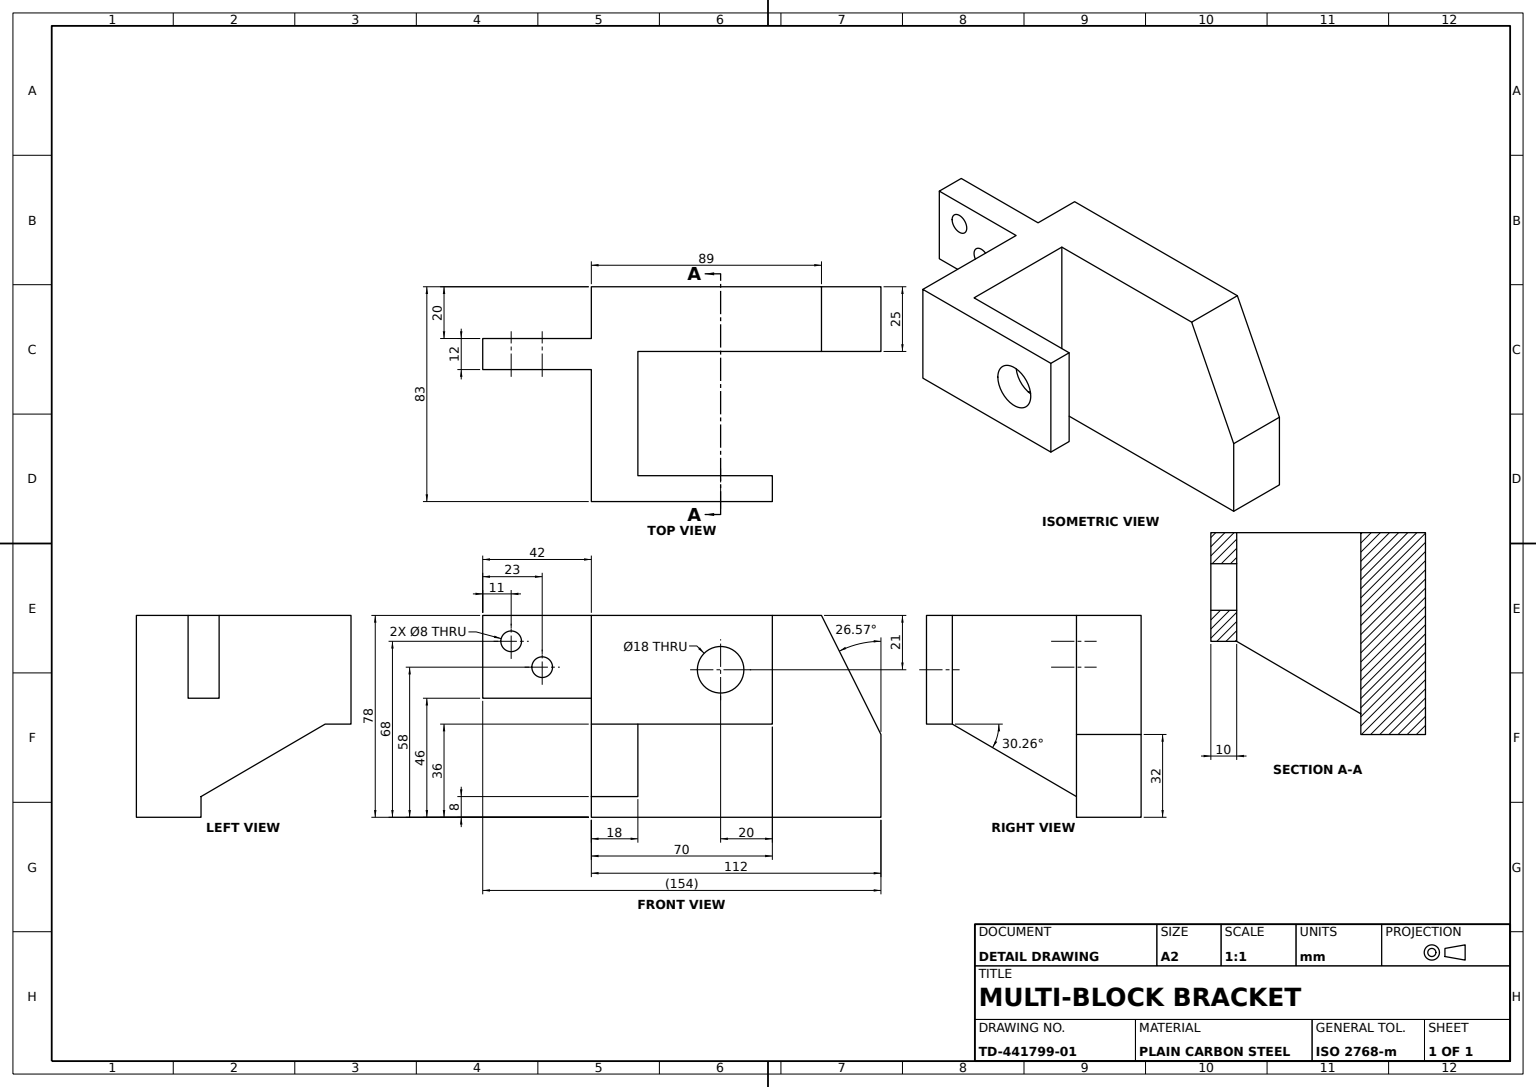
from build123d import *

# Parameters (mm, degrees)
BASE_BLOCK_DEPTH          = 25
UPRIGHT_BLOCK_DEPTH       = 18
SIDE_TAB_SKETCH_W         = 12
SIDE_TAB_SKETCH_H         = 32
SIDE_TAB_DEPTH            = 42
FRONT_PLATE_SKETCH_W      = 52
FRONT_PLATE_SKETCH_H      = 42
FRONT_PLATE_DEPTH         = 10
FRONT_PLATE_HOLE_SKETCH_R = 9
FRONT_PLATE_HOLE_DEPTH    = 10
SIDE_TAB_HOLES_SKETCH_R   = 4
SIDE_TAB_HOLES_2X_DEPTH   = 12
TRIANGULAR_GUSSET_DEPTH   = 18


with BuildPart() as part:
    # Base Block Sketch → Base Block (new body)
    with BuildSketch(Plane.XY):
        Polygon((0, 0), (112, 0), (112, 32), (89, 78), (0, 78), align=None)
    extrude(amount=BASE_BLOCK_DEPTH)

    # Upright Block Sketch → Upright Block (add)
    with BuildSketch(Plane.ZY):
        Polygon((71, 36), (25, 36), (25, 78), (83, 78), (83, 36), align=None)
    extrude(amount=-UPRIGHT_BLOCK_DEPTH)

    # Side Tab Sketch → Side Tab (add)
    with BuildSketch(Plane.ZY):
        with Locations((26, 62)):
            Rectangle(SIDE_TAB_SKETCH_W, SIDE_TAB_SKETCH_H)
    extrude(amount=SIDE_TAB_DEPTH)

    # Front Plate Sketch → Front Plate (add)
    with BuildSketch(Plane.XY.offset(83)):
        with Locations((44, 57)):
            Rectangle(FRONT_PLATE_SKETCH_W, FRONT_PLATE_SKETCH_H)
    extrude(amount=-FRONT_PLATE_DEPTH)

    # Front Plate Hole Sketch → Front Plate Hole (cut)
    with BuildSketch(Plane.XY.offset(83)):
        with Locations((50, 57)):
            Circle(FRONT_PLATE_HOLE_SKETCH_R)
    extrude(amount=-FRONT_PLATE_HOLE_DEPTH, mode=Mode.SUBTRACT)

    # Side Tab Holes Sketch → Side Tab Holes 2x (cut)
    with BuildSketch(Plane.XY.offset(32)):
        with Locations((-31, 68)):
            Circle(SIDE_TAB_HOLES_SKETCH_R)
        with Locations((-19, 58)):
            Circle(SIDE_TAB_HOLES_SKETCH_R)
    extrude(amount=-SIDE_TAB_HOLES_2X_DEPTH, mode=Mode.SUBTRACT)

    # Gusset Sketch → Triangular Gusset (add)
    with BuildSketch(Plane.ZY):
        Polygon((25, 36), (73, 36), (25, 8), align=None)
    extrude(amount=-TRIANGULAR_GUSSET_DEPTH)


solid = part.part
